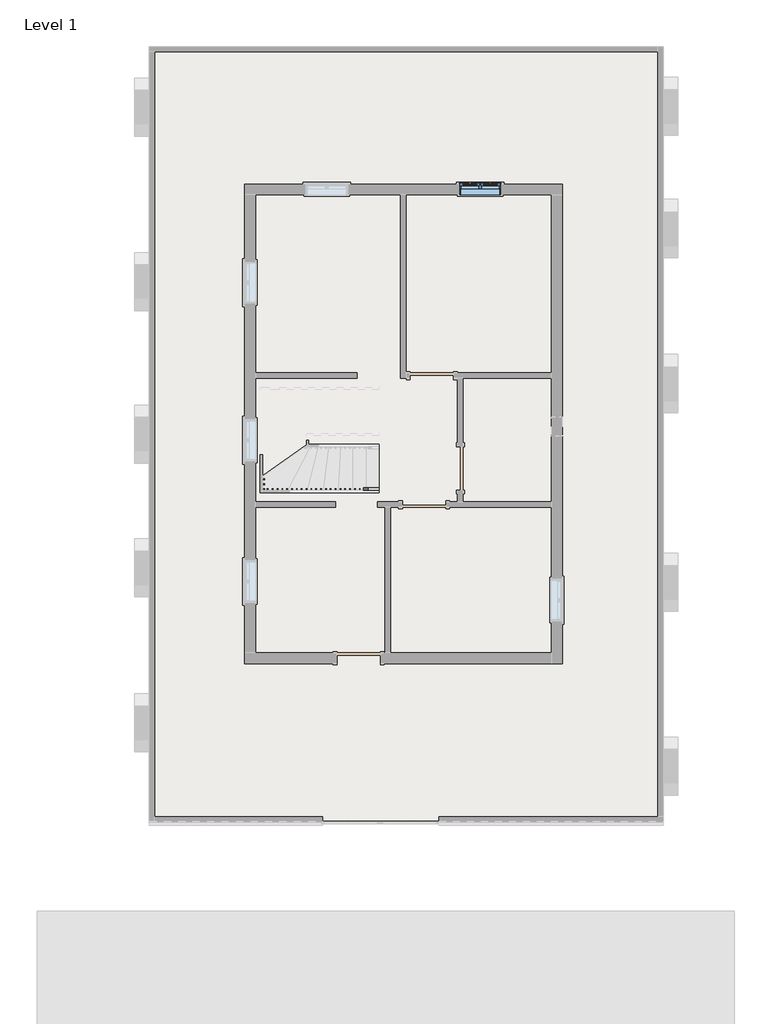
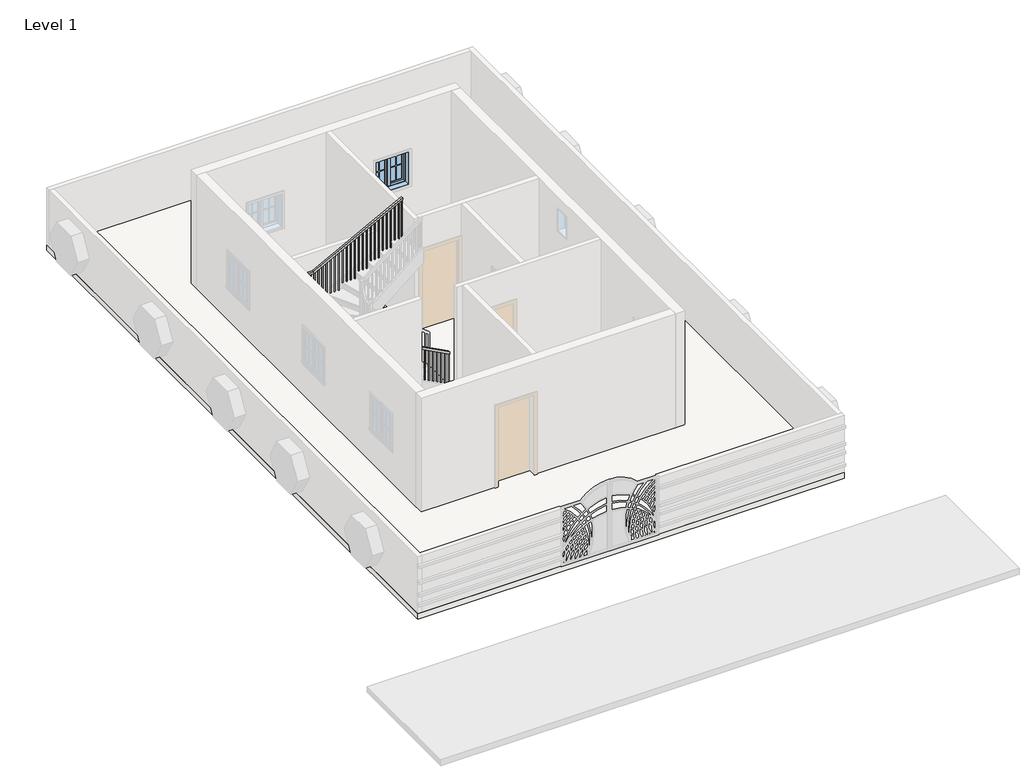
# One storey, part 2 of 3: 1 railing, 1 slab, 1 window.
"""IFC4 building model written with IfcOpenShell, lengths in millimetres."""

from ifc_helpers import new_model, si_unit, frame, origin, place, context, project, spatial, polyline, outline, extrude, faceted_brep, transform, mapped, element, save
from components import window_339605e1

model = new_model("IFC4")

# Units and contexts
model_context = context("Model", 3, world=origin())
ifc_project = project(units=[si_unit("LENGTHUNIT", "METRE", prefix="MILLI")], contexts=[model_context])

# Site, building, storey
site = spatial("IfcSite", under=ifc_project)
building = spatial("IfcBuilding", under=site)
storey = spatial("IfcBuildingStorey", under=building, Name="Level 1", Elevation=0.0)

# Railing
placement = place(None, origin())
element("IfcRailing", 1, ObjectType="Handrail - Rectangular", at=placement, inside=storey, context=model_context, shape_type="SolidModel", body=[
    faceted_brep([(-1783.4132248, -1260.1070853, 1083.7333333), (-1783.4132248, -1260.1070853, 1026.2742652), (-1783.4132248, -1209.3070853, 1026.2742652), (-1783.4132248, -1209.3070853, 1083.7333333), (-4041.1382869, -1260.1070853, 2277.0239201), (-4053.7373514, -1260.1070853, 2226.2239201), (-4053.7373514, -1209.3070853, 2226.2239201), (-4041.1382869, -1209.3070853, 2277.0239201), (-4225.5449167, -1260.1070853, 2277.0239201), (-4225.5449167, -1260.1070853, 2226.2239201), (-4174.7449167, -1209.3070853, 2226.2239201), (-4174.7449167, -1209.3070853, 2277.0239201), (-4225.5449167, -972.7952032, 2277.0239201), (-4225.5449167, -964.8446271, 2226.2239201), (-4174.7449167, -964.8446271, 2226.2239201), (-4174.7449167, -972.7952032, 2277.0239201), (-4225.5449167, 560.7810325, 2769.1094132), (-4225.5449167, 568.7316087, 2718.3094132), (-4174.7449167, 568.7316087, 2718.3094132), (-4174.7449167, 560.7810325, 2769.1094132), (-4225.5449167, 848.0929147, 2769.1094132), (-4225.5449167, 848.0929147, 2718.3094132), (-4174.7449167, 797.2929147, 2718.3094132), (-4174.7449167, 797.2929147, 2769.1094132), (-4041.1382869, 848.0929147, 2769.1094132), (-4028.5392223, 848.0929147, 2718.3094132), (-4028.5392223, 797.2929147, 2718.3094132), (-4041.1382869, 797.2929147, 2769.1094132), (-1783.4132248, 848.0929147, 3962.4), (-1783.4132248, 797.2929147, 3962.4), (-1783.4132248, 797.2929147, 3904.9409318), (-1783.4132248, 848.0929147, 3904.9409318)], [[[0, 1, 2, 3]], [[1, 0, 4, 5]], [[2, 1, 5, 6]], [[3, 2, 6, 7]], [[0, 3, 7, 4]], [[5, 4, 8, 9]], [[6, 5, 9, 10]], [[7, 6, 10, 11]], [[4, 7, 11, 8]], [[9, 8, 12, 13]], [[10, 9, 13, 14]], [[11, 10, 14, 15]], [[8, 11, 15, 12]], [[13, 12, 16, 17]], [[14, 13, 17, 18]], [[15, 14, 18, 19]], [[12, 15, 19, 16]], [[17, 16, 20, 21]], [[18, 17, 21, 22]], [[19, 18, 22, 23]], [[16, 19, 23, 20]], [[21, 20, 24, 25]], [[22, 21, 25, 26]], [[23, 22, 26, 27]], [[20, 23, 27, 24]], [[28, 29, 30, 31]], [[25, 24, 28, 31]], [[26, 25, 31, 30]], [[27, 26, 30, 29]], [[24, 27, 29, 28]]]),
    extrude(outline(polyline([(3857.6597858, -1872.8699167), (2878.6666667, -1872.8699167), (2878.6666667, -1853.8199167), (3867.7284102, -1853.8199167), (3857.6597858, -1872.8699167)])), frame((0.0, 813.1679147, 0.0), z_axis=(0.0, 1.0, 0.0), x_axis=(0.0, 0.0, 1.0)), (0.0, 0.0, 1.0), 19.05),
    extrude(outline(polyline([(3803.9604556, -1974.4699167), (2878.6666667, -1974.4699167), (2878.6666667, -1955.4199167), (3814.02908, -1955.4199167), (3803.9604556, -1974.4699167)])), frame((0.0, 813.1679147, 0.0), z_axis=(0.0, 1.0, 0.0), x_axis=(0.0, 0.0, 1.0)), (0.0, 0.0, 1.0), 19.05),
    extrude(outline(polyline([(3750.2611254, -2076.0699167), (2709.3333333, -2076.0699167), (2709.3333333, -2057.0199167), (3760.3297498, -2057.0199167), (3750.2611254, -2076.0699167)])), frame((0.0, 813.1679147, 0.0), z_axis=(0.0, 1.0, 0.0), x_axis=(0.0, 0.0, 1.0)), (0.0, 0.0, 1.0), 19.05),
    extrude(outline(polyline([(3696.5617952, -2177.6699167), (2709.3333333, -2177.6699167), (2709.3333333, -2158.6199167), (3706.6304196, -2158.6199167), (3696.5617952, -2177.6699167)])), frame((0.0, 813.1679147, 0.0), z_axis=(0.0, 1.0, 0.0), x_axis=(0.0, 0.0, 1.0)), (0.0, 0.0, 1.0), 19.05),
    extrude(outline(polyline([(3642.862465, -2279.2699167), (2709.3333333, -2279.2699167), (2709.3333333, -2260.2199167), (3652.9310894, -2260.2199167), (3642.862465, -2279.2699167)])), frame((0.0, 813.1679147, 0.0), z_axis=(0.0, 1.0, 0.0), x_axis=(0.0, 0.0, 1.0)), (0.0, 0.0, 1.0), 19.05),
    extrude(outline(polyline([(3589.1631348, -2380.8699167), (2540.0, -2380.8699167), (2540.0, -2361.8199167), (3599.2317592, -2361.8199167), (3589.1631348, -2380.8699167)])), frame((0.0, 813.1679147, 0.0), z_axis=(0.0, 1.0, 0.0), x_axis=(0.0, 0.0, 1.0)), (0.0, 0.0, 1.0), 19.05),
    extrude(outline(polyline([(3535.4638046, -2482.4699167), (2540.0, -2482.4699167), (2540.0, -2463.4199167), (3545.532429, -2463.4199167), (3535.4638046, -2482.4699167)])), frame((0.0, 813.1679147, 0.0), z_axis=(0.0, 1.0, 0.0), x_axis=(0.0, 0.0, 1.0)), (0.0, 0.0, 1.0), 19.05),
    extrude(outline(polyline([(3481.7644744, -2584.0699167), (2540.0, -2584.0699167), (2540.0, -2565.0199167), (3491.8330988, -2565.0199167), (3481.7644744, -2584.0699167)])), frame((0.0, 813.1679147, 0.0), z_axis=(0.0, 1.0, 0.0), x_axis=(0.0, 0.0, 1.0)), (0.0, 0.0, 1.0), 19.05),
    extrude(outline(polyline([(3428.0651442, -2685.6699167), (2370.6666667, -2685.6699167), (2370.6666667, -2666.6199167), (3438.1337686, -2666.6199167), (3428.0651442, -2685.6699167)])), frame((0.0, 813.1679147, 0.0), z_axis=(0.0, 1.0, 0.0), x_axis=(0.0, 0.0, 1.0)), (0.0, 0.0, 1.0), 19.05),
    extrude(outline(polyline([(3374.365814, -2787.2699167), (2370.6666667, -2787.2699167), (2370.6666667, -2768.2199167), (3384.4344384, -2768.2199167), (3374.365814, -2787.2699167)])), frame((0.0, 813.1679147, 0.0), z_axis=(0.0, 1.0, 0.0), x_axis=(0.0, 0.0, 1.0)), (0.0, 0.0, 1.0), 19.05),
    extrude(outline(polyline([(3320.6664838, -2888.8699167), (2370.6666667, -2888.8699167), (2370.6666667, -2869.8199167), (3330.7351082, -2869.8199167), (3320.6664838, -2888.8699167)])), frame((0.0, 813.1679147, 0.0), z_axis=(0.0, 1.0, 0.0), x_axis=(0.0, 0.0, 1.0)), (0.0, 0.0, 1.0), 19.05),
    extrude(outline(polyline([(3266.9671536, -2990.4699167), (2201.3333333, -2990.4699167), (2201.3333333, -2971.4199167), (3277.035778, -2971.4199167), (3266.9671536, -2990.4699167)])), frame((0.0, 813.1679147, 0.0), z_axis=(0.0, 1.0, 0.0), x_axis=(0.0, 0.0, 1.0)), (0.0, 0.0, 1.0), 19.05),
    extrude(outline(polyline([(3213.2678234, -3092.0699167), (2201.3333333, -3092.0699167), (2201.3333333, -3073.0199167), (3223.3364478, -3073.0199167), (3213.2678234, -3092.0699167)])), frame((0.0, 813.1679147, 0.0), z_axis=(0.0, 1.0, 0.0), x_axis=(0.0, 0.0, 1.0)), (0.0, 0.0, 1.0), 19.05),
    extrude(outline(polyline([(3159.5684932, -3193.6699167), (2201.3333333, -3193.6699167), (2201.3333333, -3174.6199167), (3169.6371176, -3174.6199167), (3159.5684932, -3193.6699167)])), frame((0.0, 813.1679147, 0.0), z_axis=(0.0, 1.0, 0.0), x_axis=(0.0, 0.0, 1.0)), (0.0, 0.0, 1.0), 19.05),
    extrude(outline(polyline([(3105.869163, -3295.2699167), (2201.3333333, -3295.2699167), (2201.3333333, -3276.2199167), (3115.9377874, -3276.2199167), (3105.869163, -3295.2699167)])), frame((0.0, 813.1679147, 0.0), z_axis=(0.0, 1.0, 0.0), x_axis=(0.0, 0.0, 1.0)), (0.0, 0.0, 1.0), 19.05),
    extrude(outline(polyline([(3052.1698328, -3396.8699167), (2032.0, -3396.8699167), (2032.0, -3377.8199167), (3062.2384572, -3377.8199167), (3052.1698328, -3396.8699167)])), frame((0.0, 813.1679147, 0.0), z_axis=(0.0, 1.0, 0.0), x_axis=(0.0, 0.0, 1.0)), (0.0, 0.0, 1.0), 19.05),
    extrude(outline(polyline([(2998.4705026, -3498.4699167), (2032.0, -3498.4699167), (2032.0, -3479.4199167), (3008.539127, -3479.4199167), (2998.4705026, -3498.4699167)])), frame((0.0, 813.1679147, 0.0), z_axis=(0.0, 1.0, 0.0), x_axis=(0.0, 0.0, 1.0)), (0.0, 0.0, 1.0), 19.05),
    extrude(outline(polyline([(2944.7711724, -3600.0699167), (2032.0, -3600.0699167), (2032.0, -3581.0199167), (2954.8397968, -3581.0199167), (2944.7711724, -3600.0699167)])), frame((0.0, 813.1679147, 0.0), z_axis=(0.0, 1.0, 0.0), x_axis=(0.0, 0.0, 1.0)), (0.0, 0.0, 1.0), 19.05),
    extrude(outline(polyline([(2891.0718422, -3701.6699167), (2032.0, -3701.6699167), (2032.0, -3682.6199167), (2901.1404666, -3682.6199167), (2891.0718422, -3701.6699167)])), frame((0.0, 813.1679147, 0.0), z_axis=(0.0, 1.0, 0.0), x_axis=(0.0, 0.0, 1.0)), (0.0, 0.0, 1.0), 19.05),
    extrude(outline(polyline([(2837.372512, -3803.2699167), (1862.6666667, -3803.2699167), (1862.6666667, -3784.2199167), (2847.4411364, -3784.2199167), (2837.372512, -3803.2699167)])), frame((0.0, 813.1679147, 0.0), z_axis=(0.0, 1.0, 0.0), x_axis=(0.0, 0.0, 1.0)), (0.0, 0.0, 1.0), 19.05),
    extrude(outline(polyline([(2783.6731818, -3904.8699167), (1862.6666667, -3904.8699167), (1862.6666667, -3885.8199167), (2793.7418062, -3885.8199167), (2783.6731818, -3904.8699167)])), frame((0.0, 813.1679147, 0.0), z_axis=(0.0, 1.0, 0.0), x_axis=(0.0, 0.0, 1.0)), (0.0, 0.0, 1.0), 19.05),
    extrude(outline(polyline([(2729.9738516, -4006.4699167), (1862.6666667, -4006.4699167), (1862.6666667, -3987.4199167), (2740.042476, -3987.4199167), (2729.9738516, -4006.4699167)])), frame((0.0, 813.1679147, 0.0), z_axis=(0.0, 1.0, 0.0), x_axis=(0.0, 0.0, 1.0)), (0.0, 0.0, 1.0), 19.05),
    extrude(outline(polyline([(-4108.0699167, 832.2179147), (-4089.0199167, 832.2179147), (-4089.0199167, 813.1679147), (-4108.0699167, 813.1679147), (-4108.0699167, 832.2179147)])), frame((0.0, 0.0, 1862.6666667), z_axis=(0.0, 0.0, 1.0), x_axis=(1.0, 0.0, 0.0)), (0.0, 0.0, 1.0), 855.6427466),
    extrude(outline(polyline([(-4209.6699167, 787.7679147), (-4209.6699167, 806.8179147), (-4190.6199167, 806.8179147), (-4190.6199167, 787.7679147), (-4209.6699167, 787.7679147)])), frame((0.0, 0.0, 1862.6666667), z_axis=(0.0, 0.0, 1.0), x_axis=(1.0, 0.0, 0.0)), (0.0, 0.0, 1.0), 855.6427466),
    extrude(outline(polyline([(-4209.6699167, 686.1679147), (-4209.6699167, 705.2179147), (-4190.6199167, 705.2179147), (-4190.6199167, 686.1679147), (-4209.6699167, 686.1679147)])), frame((0.0, 0.0, 1862.6666667), z_axis=(0.0, 0.0, 1.0), x_axis=(1.0, 0.0, 0.0)), (0.0, 0.0, 1.0), 855.6427466),
    extrude(outline(polyline([(-4209.6699167, 584.5679147), (-4209.6699167, 603.6179147), (-4190.6199167, 603.6179147), (-4190.6199167, 584.5679147), (-4209.6699167, 584.5679147)])), frame((0.0, 0.0, 1862.6666667), z_axis=(0.0, 0.0, 1.0), x_axis=(1.0, 0.0, 0.0)), (0.0, 0.0, 1.0), 855.6427466),
    extrude(outline(polyline([(502.0179147, 2696.9026907), (502.0179147, 1693.3333333), (482.9679147, 1693.3333333), (482.9679147, 2690.7900316), (502.0179147, 2696.9026907)])), frame((-4209.6699167, 0.0, 0.0), z_axis=(1.0, 0.0, 0.0), x_axis=(0.0, 1.0, 0.0)), (0.0, 0.0, 1.0), 19.05),
    extrude(outline(polyline([(400.4179147, 2664.3018425), (400.4179147, 1693.3333333), (381.3679147, 1693.3333333), (381.3679147, 2658.1891834), (400.4179147, 2664.3018425)])), frame((-4209.6699167, 0.0, 0.0), z_axis=(1.0, 0.0, 0.0), x_axis=(0.0, 1.0, 0.0)), (0.0, 0.0, 1.0), 19.05),
    extrude(outline(polyline([(298.8179147, 2631.7009942), (298.8179147, 1693.3333333), (279.7679147, 1693.3333333), (279.7679147, 2625.5883352), (298.8179147, 2631.7009942)])), frame((-4209.6699167, 0.0, 0.0), z_axis=(1.0, 0.0, 0.0), x_axis=(0.0, 1.0, 0.0)), (0.0, 0.0, 1.0), 19.05),
    extrude(outline(polyline([(197.2179147, 2599.100146), (197.2179147, 1693.3333333), (178.1679147, 1693.3333333), (178.1679147, 2592.987487), (197.2179147, 2599.100146)])), frame((-4209.6699167, 0.0, 0.0), z_axis=(1.0, 0.0, 0.0), x_axis=(0.0, 1.0, 0.0)), (0.0, 0.0, 1.0), 19.05),
    extrude(outline(polyline([(95.6179147, 2566.4992978), (95.6179147, 1693.3333333), (76.5679147, 1693.3333333), (76.5679147, 2560.3866387), (95.6179147, 2566.4992978)])), frame((-4209.6699167, 0.0, 0.0), z_axis=(1.0, 0.0, 0.0), x_axis=(0.0, 1.0, 0.0)), (0.0, 0.0, 1.0), 19.05),
    extrude(outline(polyline([(-5.9820853, 2533.8984495), (-5.9820853, 1524.0), (-25.0320853, 1524.0), (-25.0320853, 2527.7857905), (-5.9820853, 2533.8984495)])), frame((-4209.6699167, 0.0, 0.0), z_axis=(1.0, 0.0, 0.0), x_axis=(0.0, 1.0, 0.0)), (0.0, 0.0, 1.0), 19.05),
    extrude(outline(polyline([(-107.5820853, 2501.2976013), (-107.5820853, 1524.0), (-126.6320853, 1524.0), (-126.6320853, 2495.1849423), (-107.5820853, 2501.2976013)])), frame((-4209.6699167, 0.0, 0.0), z_axis=(1.0, 0.0, 0.0), x_axis=(0.0, 1.0, 0.0)), (0.0, 0.0, 1.0), 19.05),
    extrude(outline(polyline([(-209.1820853, 2468.6967531), (-209.1820853, 1524.0), (-228.2320853, 1524.0), (-228.2320853, 2462.5840941), (-209.1820853, 2468.6967531)])), frame((-4209.6699167, 0.0, 0.0), z_axis=(1.0, 0.0, 0.0), x_axis=(0.0, 1.0, 0.0)), (0.0, 0.0, 1.0), 19.05),
    extrude(outline(polyline([(-310.7820853, 2436.0959049), (-310.7820853, 1524.0), (-329.8320853, 1524.0), (-329.8320853, 2429.9832458), (-310.7820853, 2436.0959049)])), frame((-4209.6699167, 0.0, 0.0), z_axis=(1.0, 0.0, 0.0), x_axis=(0.0, 1.0, 0.0)), (0.0, 0.0, 1.0), 19.05),
    extrude(outline(polyline([(-412.3820853, 2403.4950566), (-412.3820853, 1524.0), (-431.4320853, 1524.0), (-431.4320853, 2397.3823976), (-412.3820853, 2403.4950566)])), frame((-4209.6699167, 0.0, 0.0), z_axis=(1.0, 0.0, 0.0), x_axis=(0.0, 1.0, 0.0)), (0.0, 0.0, 1.0), 19.05),
    extrude(outline(polyline([(-513.9820853, 2370.8942084), (-513.9820853, 1354.6666667), (-533.0320853, 1354.6666667), (-533.0320853, 2364.7815494), (-513.9820853, 2370.8942084)])), frame((-4209.6699167, 0.0, 0.0), z_axis=(1.0, 0.0, 0.0), x_axis=(0.0, 1.0, 0.0)), (0.0, 0.0, 1.0), 19.05),
    extrude(outline(polyline([(-615.5820853, 2338.2933602), (-615.5820853, 1354.6666667), (-634.6320853, 1354.6666667), (-634.6320853, 2332.1807011), (-615.5820853, 2338.2933602)])), frame((-4209.6699167, 0.0, 0.0), z_axis=(1.0, 0.0, 0.0), x_axis=(0.0, 1.0, 0.0)), (0.0, 0.0, 1.0), 19.05),
    extrude(outline(polyline([(-717.1820853, 2305.692512), (-717.1820853, 1354.6666667), (-736.2320853, 1354.6666667), (-736.2320853, 2299.5798529), (-717.1820853, 2305.692512)])), frame((-4209.6699167, 0.0, 0.0), z_axis=(1.0, 0.0, 0.0), x_axis=(0.0, 1.0, 0.0)), (0.0, 0.0, 1.0), 19.05),
    extrude(outline(polyline([(-818.7820853, 2273.0916637), (-818.7820853, 1354.6666667), (-837.8320853, 1354.6666667), (-837.8320853, 2266.9790047), (-818.7820853, 2273.0916637)])), frame((-4209.6699167, 0.0, 0.0), z_axis=(1.0, 0.0, 0.0), x_axis=(0.0, 1.0, 0.0)), (0.0, 0.0, 1.0), 19.05),
    extrude(outline(polyline([(-920.3820853, 2240.4908155), (-920.3820853, 1354.6666667), (-939.4320853, 1354.6666667), (-939.4320853, 2234.3781565), (-920.3820853, 2240.4908155)])), frame((-4209.6699167, 0.0, 0.0), z_axis=(1.0, 0.0, 0.0), x_axis=(0.0, 1.0, 0.0)), (0.0, 0.0, 1.0), 19.05),
    extrude(outline(polyline([(-4209.6699167, -1041.0320853), (-4209.6699167, -1021.9820853), (-4190.6199167, -1021.9820853), (-4190.6199167, -1041.0320853), (-4209.6699167, -1041.0320853)])), frame((0.0, 0.0, 1185.3333333), z_axis=(0.0, 0.0, 1.0), x_axis=(1.0, 0.0, 0.0)), (0.0, 0.0, 1.0), 1040.8905868),
    extrude(outline(polyline([(-4209.6699167, -1142.6320853), (-4209.6699167, -1123.5820853), (-4190.6199167, -1123.5820853), (-4190.6199167, -1142.6320853), (-4209.6699167, -1142.6320853)])), frame((0.0, 0.0, 1185.3333333), z_axis=(0.0, 0.0, 1.0), x_axis=(1.0, 0.0, 0.0)), (0.0, 0.0, 1.0), 1040.8905868),
    extrude(outline(polyline([(-4110.6882248, -1244.2320853), (-4129.7382248, -1244.2320853), (-4129.7382248, -1225.1820853), (-4110.6882248, -1225.1820853), (-4110.6882248, -1244.2320853)])), frame((0.0, 0.0, 1185.3333333), z_axis=(0.0, 0.0, 1.0), x_axis=(1.0, 0.0, 0.0)), (0.0, 0.0, 1.0), 1040.8905868),
    extrude(outline(polyline([(2212.6938418, -4028.1382248), (1185.3333333, -4028.1382248), (1185.3333333, -4009.0882248), (2202.6252174, -4009.0882248), (2212.6938418, -4028.1382248)])), frame((0.0, -1244.2320853, 0.0), z_axis=(0.0, 1.0, 0.0), x_axis=(0.0, 0.0, 1.0)), (0.0, 0.0, 1.0), 19.05),
    extrude(outline(polyline([(2158.9945116, -3926.5382248), (1185.3333333, -3926.5382248), (1185.3333333, -3907.4882248), (2148.9258872, -3907.4882248), (2158.9945116, -3926.5382248)])), frame((0.0, -1244.2320853, 0.0), z_axis=(0.0, 1.0, 0.0), x_axis=(0.0, 0.0, 1.0)), (0.0, 0.0, 1.0), 19.05),
    extrude(outline(polyline([(2105.2951814, -3824.9382248), (1185.3333333, -3824.9382248), (1185.3333333, -3805.8882248), (2095.226557, -3805.8882248), (2105.2951814, -3824.9382248)])), frame((0.0, -1244.2320853, 0.0), z_axis=(0.0, 1.0, 0.0), x_axis=(0.0, 0.0, 1.0)), (0.0, 0.0, 1.0), 19.05),
    extrude(outline(polyline([(2051.5958512, -3723.3382248), (1185.3333333, -3723.3382248), (1185.3333333, -3704.2882248), (2041.5272268, -3704.2882248), (2051.5958512, -3723.3382248)])), frame((0.0, -1244.2320853, 0.0), z_axis=(0.0, 1.0, 0.0), x_axis=(0.0, 0.0, 1.0)), (0.0, 0.0, 1.0), 19.05),
    extrude(outline(polyline([(1997.896521, -3621.7382248), (1016.0, -3621.7382248), (1016.0, -3602.6882248), (1987.8278966, -3602.6882248), (1997.896521, -3621.7382248)])), frame((0.0, -1244.2320853, 0.0), z_axis=(0.0, 1.0, 0.0), x_axis=(0.0, 0.0, 1.0)), (0.0, 0.0, 1.0), 19.05),
    extrude(outline(polyline([(1944.1971908, -3520.1382248), (1016.0, -3520.1382248), (1016.0, -3501.0882248), (1934.1285664, -3501.0882248), (1944.1971908, -3520.1382248)])), frame((0.0, -1244.2320853, 0.0), z_axis=(0.0, 1.0, 0.0), x_axis=(0.0, 0.0, 1.0)), (0.0, 0.0, 1.0), 19.05),
    extrude(outline(polyline([(1890.4978606, -3418.5382248), (1016.0, -3418.5382248), (1016.0, -3399.4882248), (1880.4292362, -3399.4882248), (1890.4978606, -3418.5382248)])), frame((0.0, -1244.2320853, 0.0), z_axis=(0.0, 1.0, 0.0), x_axis=(0.0, 0.0, 1.0)), (0.0, 0.0, 1.0), 19.05),
    extrude(outline(polyline([(1836.7985304, -3316.9382248), (1016.0, -3316.9382248), (1016.0, -3297.8882248), (1826.729906, -3297.8882248), (1836.7985304, -3316.9382248)])), frame((0.0, -1244.2320853, 0.0), z_axis=(0.0, 1.0, 0.0), x_axis=(0.0, 0.0, 1.0)), (0.0, 0.0, 1.0), 19.05),
    extrude(outline(polyline([(1783.0992002, -3215.3382248), (846.6666667, -3215.3382248), (846.6666667, -3196.2882248), (1773.0305758, -3196.2882248), (1783.0992002, -3215.3382248)])), frame((0.0, -1244.2320853, 0.0), z_axis=(0.0, 1.0, 0.0), x_axis=(0.0, 0.0, 1.0)), (0.0, 0.0, 1.0), 19.05),
    extrude(outline(polyline([(1729.39987, -3113.7382248), (846.6666667, -3113.7382248), (846.6666667, -3094.6882248), (1719.3312456, -3094.6882248), (1729.39987, -3113.7382248)])), frame((0.0, -1244.2320853, 0.0), z_axis=(0.0, 1.0, 0.0), x_axis=(0.0, 0.0, 1.0)), (0.0, 0.0, 1.0), 19.05),
    extrude(outline(polyline([(1675.7005398, -3012.1382248), (846.6666667, -3012.1382248), (846.6666667, -2993.0882248), (1665.6319154, -2993.0882248), (1675.7005398, -3012.1382248)])), frame((0.0, -1244.2320853, 0.0), z_axis=(0.0, 1.0, 0.0), x_axis=(0.0, 0.0, 1.0)), (0.0, 0.0, 1.0), 19.05),
    extrude(outline(polyline([(1622.0012096, -2910.5382248), (677.3333333, -2910.5382248), (677.3333333, -2891.4882248), (1611.9325852, -2891.4882248), (1622.0012096, -2910.5382248)])), frame((0.0, -1244.2320853, 0.0), z_axis=(0.0, 1.0, 0.0), x_axis=(0.0, 0.0, 1.0)), (0.0, 0.0, 1.0), 19.05),
    extrude(outline(polyline([(1568.3018794, -2808.9382248), (677.3333333, -2808.9382248), (677.3333333, -2789.8882248), (1558.233255, -2789.8882248), (1568.3018794, -2808.9382248)])), frame((0.0, -1244.2320853, 0.0), z_axis=(0.0, 1.0, 0.0), x_axis=(0.0, 0.0, 1.0)), (0.0, 0.0, 1.0), 19.05),
    extrude(outline(polyline([(1514.6025492, -2707.3382248), (677.3333333, -2707.3382248), (677.3333333, -2688.2882248), (1504.5339248, -2688.2882248), (1514.6025492, -2707.3382248)])), frame((0.0, -1244.2320853, 0.0), z_axis=(0.0, 1.0, 0.0), x_axis=(0.0, 0.0, 1.0)), (0.0, 0.0, 1.0), 19.05),
    extrude(outline(polyline([(1460.903219, -2605.7382248), (508.0, -2605.7382248), (508.0, -2586.6882248), (1450.8345946, -2586.6882248), (1460.903219, -2605.7382248)])), frame((0.0, -1244.2320853, 0.0), z_axis=(0.0, 1.0, 0.0), x_axis=(0.0, 0.0, 1.0)), (0.0, 0.0, 1.0), 19.05),
    extrude(outline(polyline([(1407.2038888, -2504.1382248), (508.0, -2504.1382248), (508.0, -2485.0882248), (1397.1352644, -2485.0882248), (1407.2038888, -2504.1382248)])), frame((0.0, -1244.2320853, 0.0), z_axis=(0.0, 1.0, 0.0), x_axis=(0.0, 0.0, 1.0)), (0.0, 0.0, 1.0), 19.05),
    extrude(outline(polyline([(1353.5045586, -2402.5382248), (508.0, -2402.5382248), (508.0, -2383.4882248), (1343.4359342, -2383.4882248), (1353.5045586, -2402.5382248)])), frame((0.0, -1244.2320853, 0.0), z_axis=(0.0, 1.0, 0.0), x_axis=(0.0, 0.0, 1.0)), (0.0, 0.0, 1.0), 19.05),
    extrude(outline(polyline([(1299.8052284, -2300.9382248), (338.6666667, -2300.9382248), (338.6666667, -2281.8882248), (1289.736604, -2281.8882248), (1299.8052284, -2300.9382248)])), frame((0.0, -1244.2320853, 0.0), z_axis=(0.0, 1.0, 0.0), x_axis=(0.0, 0.0, 1.0)), (0.0, 0.0, 1.0), 19.05),
    extrude(outline(polyline([(1246.1058982, -2199.3382248), (338.6666667, -2199.3382248), (338.6666667, -2180.2882248), (1236.0372738, -2180.2882248), (1246.1058982, -2199.3382248)])), frame((0.0, -1244.2320853, 0.0), z_axis=(0.0, 1.0, 0.0), x_axis=(0.0, 0.0, 1.0)), (0.0, 0.0, 1.0), 19.05),
    extrude(outline(polyline([(1192.406568, -2097.7382248), (338.6666667, -2097.7382248), (338.6666667, -2078.6882248), (1182.3379436, -2078.6882248), (1192.406568, -2097.7382248)])), frame((0.0, -1244.2320853, 0.0), z_axis=(0.0, 1.0, 0.0), x_axis=(0.0, 0.0, 1.0)), (0.0, 0.0, 1.0), 19.05),
    extrude(outline(polyline([(1138.7072378, -1996.1382248), (169.3333333, -1996.1382248), (169.3333333, -1977.0882248), (1128.6386134, -1977.0882248), (1138.7072378, -1996.1382248)])), frame((0.0, -1244.2320853, 0.0), z_axis=(0.0, 1.0, 0.0), x_axis=(0.0, 0.0, 1.0)), (0.0, 0.0, 1.0), 19.05),
    extrude(outline(polyline([(1085.0079076, -1894.5382248), (169.3333333, -1894.5382248), (169.3333333, -1875.4882248), (1074.9392831, -1875.4882248), (1085.0079076, -1894.5382248)])), frame((0.0, -1244.2320853, 0.0), z_axis=(0.0, 1.0, 0.0), x_axis=(0.0, 0.0, 1.0)), (0.0, 0.0, 1.0), 19.05),
    extrude(outline(polyline([(-4209.6699167, 813.1679147), (-4209.6699167, 832.2179147), (-4190.6199167, 832.2179147), (-4190.6199167, 813.1679147), (-4209.6699167, 813.1679147)])), frame((0.0, 0.0, 1862.6666667), z_axis=(0.0, 0.0, 1.0), x_axis=(1.0, 0.0, 0.0)), (0.0, 0.0, 1.0), 855.6427466),
    extrude(outline(polyline([(-4190.6199167, -1244.2320853), (-4209.6699167, -1244.2320853), (-4209.6699167, -1225.1820853), (-4190.6199167, -1225.1820853), (-4190.6199167, -1244.2320853)])), frame((0.0, 0.0, 1185.3333333), z_axis=(0.0, 0.0, 1.0), x_axis=(1.0, 0.0, 0.0)), (0.0, 0.0, 1.0), 1040.8905868),
    extrude(outline(polyline([(3894.8723074, -1802.4632248), (2878.6666667, -1802.4632248), (2878.6666667, -1783.4132248), (3904.9409318, -1783.4132248), (3894.8723074, -1802.4632248)])), frame((0.0, 813.1679147, 0.0), z_axis=(0.0, 1.0, 0.0), x_axis=(0.0, 0.0, 1.0)), (0.0, 0.0, 1.0), 19.05),
    extrude(outline(polyline([(1036.3428896, -1802.4632248), (169.3333333, -1802.4632248), (169.3333333, -1783.4132248), (1026.2742652, -1783.4132248), (1036.3428896, -1802.4632248)])), frame((0.0, -1244.2320853, 0.0), z_axis=(0.0, 1.0, 0.0), x_axis=(0.0, 0.0, 1.0)), (0.0, 0.0, 1.0), 19.05),
])

# Slab
element("IfcSlab", 2, ObjectType="Generic - 12\"", at=placement, inside=storey, context=model_context, shape_type="SweptSolid", body=[
    extrude(outline(polyline([(4175.6127609, 8043.4943296), (4175.6127609, -8225.2056704), (-6606.6872391, -8225.2056704), (-6606.6872391, 8043.4943296), (4175.6127609, 8043.4943296)])), frame((0.0, 0.0, -152.4), z_axis=(0.0, 0.0, 1.0), x_axis=(1.0, 0.0, 0.0)), (0.0, 0.0, 1.0), 152.4),
])

# Window
window_shape = window_339605e1(model_context)
element("IfcWindow", 3, ObjectType="Window-Casement-Double : 34\" x 36\"", at=placement, inside=storey, context=model_context, shape_type="MappedRepresentation", body=[
    mapped(window_shape, transform((336.9300833, 5045.4429147, 0.0), x_axis=(1.0, 0.0, 0.0), y_axis=(0.0, 1.0, 0.0), z_axis=(0.0, 0.0, 1.0))),
])

save(model, "model.ifc")

# Revit data of these elements
# Type "Handrail - Rectangular"
#   Assembly Code = "C2010400"
#   built-in parameter 1008612 = 0.0416667 (stored number, unit not read)
#   built-in parameter 1008611 = 0.0416667 (stored number, unit not read)
#   built-in parameter 1008609 = 0.333333 (stored number, unit not read)
#   built-in parameter 1008604 = 0.166667 (stored number, unit not read)
#   built-in parameter 1008603 = 0.166667 (stored number, unit not read)
#   Railing Height = 3' - 0"
#   built-in parameter 1008630 = 2
#   built-in parameter 1008610 = 2
#   built-in parameter 1008618 = Baluster - Square : 3/4"
# Type "Generic - 12\""
#   Assembly Code = "B1010"
#   Function = 0
#   Layers, outside or top first: 0' - 6" no material (function 1)
# Type "Window-Casement-Double : 34\" x 36\""
#   Type Mark = "14"
#   Fire Rating = "0.5h"
#   Assembly Code = "B2020100"
#   Analytic Construction = "Double glazing - domestic"
#   Frame Extension [instance default] = 0' - 0 1/4"
#   Window Inset [instance default] = 0' - 0"
#   Wall Thickness [instance default] = 0' - 6"
#   Interior Wall Closure [instance default] = 0' - 2 1/4"
#   Half Width = 1' - 5"
#   Visual Light Transmittance = 0.81
#   Thermal Resistance (R) = 1.8146 (h·ft²·°F)/BTU
#   Solar Heat Gain Coefficient = 0.76
#   Rough Width = 2' - 10 1/2"
#   Rough Height = 3' - 0 1/2"
#   Height = 3' - 0"
#   Heat Transfer Coefficient (U) = 0.5511 BTU/(h·ft²·°F)
#   Exterior Wall Closure [instance default] = 0' - 1 1/4"
#   Extension Jamb [instance default] = 0' - 2 1/4"
#   Default Sill Height = 3' - 0"
#   Width = 2' - 10"
#   Define Thermal Properties by = 0
#   Muntin Visibility = yes
#   Interior Trim Visibility [instance default] = yes
#   Exterior Trim Visibility [instance default] = yes
#   Extension Jamb Visibility [instance default] = yes
#   Interior Trim Material = Wood - Stained
#   Muntin Pattern = Muntin Pattern_2x2 : Muntin Pattern_2x2
#   Interior Trim = Trim-Window-Interior-Flat : Picture Frame
#   Interior Frame Material = Wood - Stained
#   Glass Panel Material = Glass
#   Exterior Trim Material = Clad - White
#   Exterior Trim = Trim-Window-Exterior-Flat : with Sill
#   Exterior Frame Material = Clad - White
#   Wall Closure = (empty or 0)
# Element 1 (IfcRailing, "Handrail - Rectangular")
#   Phase Created = New Construction
# Element 2 (IfcSlab, "Generic - 12\"")
#   Height Offset From Level = 0' - 0"
#   Phase Created = New Construction
#   Materials on its faces: "Default Floor"
# Element 3 (IfcWindow, "Window-Casement-Double : 34\" x 36\"")
#   Mark = "3"
#   Window Inset = 0' - 0"
#   Interior Wall Closure = 0' - 2 1/4"
#   Frame Extension = 0' - 0 1/4"
#   Exterior Wall Closure = 0' - 1 1/4"
#   Interior Trim Visibility = yes
#   Exterior Trim Visibility = yes
#   Phase Created = New Construction
#   Materials on its faces: "Wood - Stained", "Glass", "Clad - White"
# Materials
#   "Wood - Stained": class "Wood", colour RGB 224 178 126, transparency 0, Cost = 0
#   "Glass": class "Glass", colour RGB 0 128 192, transparency 0.75, Description = "Soda Lime Glass", Cost = 0
#   "Clad - White": class "Wood", colour RGB 242 242 238, transparency 0, Cost = 0
#   "Default Floor": colour RGB 128 128 128, transparency 0, Cost = 0
